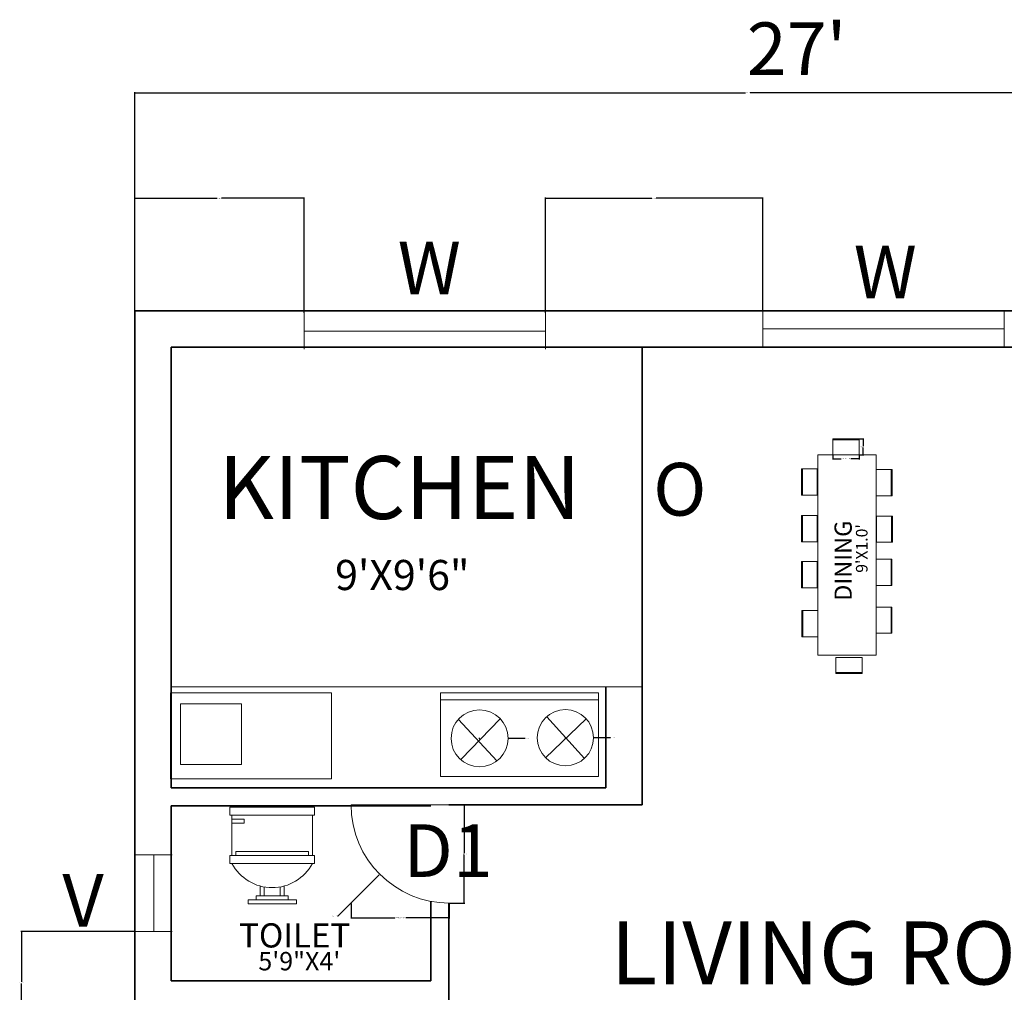
# Model space of a CAD drawing. Units: inches. Extents: x -26 to 788, y -42 to 505.
# Tile 5 of 9: x -26 to 219, y 262 to 504. Entities that reach past the tile are written whole.
import ezdxf

# ---------------------------------------------------------------- set-up
doc = ezdxf.new("R2010")
doc.units = ezdxf.units.IN
doc.header["$MEASUREMENT"] = 0
for name, color, linetype, lineweight in [('A-ANNO-DIMS', 2, 'Continuous', 18), ('A-ANNO-IDEN', 3, 'Continuous', 18), ('A-AREA-IDEN', 7, 'Continuous', 18), ('A-DOOR', 3, 'Continuous', 18), ('A-EQPM', 8, 'Continuous', 18), ('A-FLOR-FIXT', 9, 'Continuous', 18), ('A-FURN', 8, 'Continuous', 18), ('A-GLAZ', 4, 'Continuous', 18), ('A-WALL', 7, 'Continuous', 35)]:
    doc.layers.add(name, color=color, linetype=linetype, lineweight=lineweight)
doc.styles.get("Standard").update_dxf_attribs({"font": 'arial.ttf'})
doc.dimstyles.get("Standard").update_dxf_attribs({"dimtxt": 0.18, "dimasz": 0.18, "dimexe": 0.18, "dimexo": 0.0625, "dimgap": 0.09, "dimtad": 0, "dimtih": 1, "dimtoh": 1, "dimdec": 4, "dimzin": 0, "dimdsep": 46, "dimtxsty": 'Standard', "dimcen": 0.09, "dimadec": 0, "dimazin": 0, "dimtfac": 1, "dimtdec": 4, "dimtofl": 0, "dimtmove": 0, "dimatfit": 3, "dimfxl": 1, "dimtolj": 1, "dimtzin": 0, "dimarcsym": 0})

# ---------------------------------------------------------------- blocks, each defined once
blk = doc.blocks.new('*U2')
for p, q in [((-10, 22), (-10, 12)), ((-10, 21), (-7, 21)), ((-7, 20), (-10, 20)), ((-7, 21), (-7, 20)), ((10, 12), (10, 22)), ((9, 13), (-9, 13)), ((-9, 13), (-9, 12)), ((9, 12), (9, 13)), ((10.5, 12), (-10.5, 12)), ((-10.5, 10), (-10.5, 12)), ((10.5, 10), (-10.5, 10)), ((10.5, 12), (10.5, 10)), ((-3, 4.4065), (-3, 2)), ((-2, 2), (-2, 4.1658)), ((2, 4.1658), (2, 2)), ((3, 2), (3, 4.4065)), ((4, 2), (-4, 2)), ((-4, 2), (-4, 1)), ((4, 1), (4, 2))]:
    blk.add_line(p, q)
for points in [[(10.5, 22), (10.5, 24), (-10.5, 24), (-10.5, 22)], [(6, 0), (6, 1), (-6, 1), (-6, 0)]]:
    blk.add_lwpolyline(points, close=True)
blk.add_arc((0, 15.3333), 11.3333, 208.0725, 331.9275)
blk = doc.blocks.new('*D7')
at = {"layer": 'A-ANNO-DIMS', "color": 0, "lineweight": -2, "transparency": 16777216}
for p, q in [((2.95, 431.18), (2.95, 485.53)), ((3.13, 485.35), (154.6, 485.35)), ((307.27, 485.35), (155.81, 485.35)), ((307.45, 431.18), (307.45, 485.53))]:
    blk.add_line(p, q, dxfattribs=at)
at = {"layer": 'A-ANNO-DIMS', "color": 0, "transparency": 16777216}
for points in [[(3.13, 485.38), (3.13, 485.32), (2.95, 485.35)], [(307.27, 485.38), (307.27, 485.32), (307.45, 485.35)]]:
    blk.add_solid(points, dxfattribs=at)
at = {"layer": 'Defpoints', "color": 0, "transparency": 16777216}
for p in [(307.45, 485.35), (2.95, 431.12), (307.45, 431.12)]:
    blk.add_point(p, dxfattribs=at)
at = {"layer": 'A-ANNO-DIMS', "color": 0, "transparency": 16777216, "insert": (155.2, 485.35), "char_height": 0.18, "attachment_point": 5}
blk.add_mtext('\\A1;304.5000', dxfattribs=at)
blk = doc.blocks.new('WIN-SLIDER-60')
for p, q in [((0, 9), (0, 0)), ((60, 9), (60, 0)), ((0, 4.5), (60, 4.5)), ((60, 4.5), (50.65, 4.5))]:
    blk.add_line(p, q)
blk = doc.blocks.new('VENT-BATH')
for p, q in [((9, 19.08), (0, 19.08)), ((4.5, 19.08), (4.5, 0)), ((9, 0), (0, 0))]:
    blk.add_line(p, q)
blk = doc.blocks.new('DOOR-BATH-B')
blk.add_line((24.41, 24.41), (0, 24.41))
blk.add_arc((24.41, 24.41), 24.41, 180, 270)
blk = doc.blocks.new('CHAIR-DINING')
for points in [[(0, 3.72), (6.52, 3.72), (6.52, 3.95), (0, 3.95)], [(0, 0), (6.52, 0), (6.52, 3.72), (0, 3.72)]]:
    blk.add_lwpolyline(points, close=True)
blk = doc.blocks.new('*D25')
at = {"layer": 'A-ANNO-DIMS', "color": 0, "lineweight": -2, "transparency": 16777216}
for p, q in [((176.36, 395.3), (176.36, 394.21)), ((176.54, 394.39), (178.43, 394.39)), ((182.71, 394.39), (180.82, 394.39)), ((182.89, 395.3), (182.89, 394.21))]:
    blk.add_line(p, q, dxfattribs=at)
at = {"layer": 'A-ANNO-DIMS', "color": 0, "transparency": 16777216}
for points in [[(176.54, 394.42), (176.54, 394.36), (176.36, 394.39)], [(182.71, 394.42), (182.71, 394.36), (182.89, 394.39)]]:
    blk.add_solid(points, dxfattribs=at)
at = {"layer": 'Defpoints', "color": 0, "transparency": 16777216}
for p in [(176.36, 395.37), (182.89, 395.37), (182.89, 394.39)]:
    blk.add_point(p, dxfattribs=at)
at = {"layer": 'A-ANNO-DIMS', "color": 0, "transparency": 16777216, "insert": (179.62, 394.39), "char_height": 0.18, "attachment_point": 5}
blk.add_mtext('\\A1;CHAIR 6.5246 TYP.', dxfattribs=at)
blk = doc.blocks.new('*D26')
at = {"layer": 'A-ANNO-DIMS', "color": 0, "lineweight": -2, "transparency": 16777216}
for p, q in [((182.95, 399.32), (184.04, 399.32)), ((183.86, 399.14), (183.86, 397.52)), ((183.86, 395.55), (183.86, 397.16)), ((182.95, 395.37), (184.04, 395.37))]:
    blk.add_line(p, q, dxfattribs=at)
at = {"layer": 'A-ANNO-DIMS', "color": 0, "transparency": 16777216}
for points in [[(183.83, 399.14), (183.89, 399.14), (183.86, 399.32)], [(183.83, 395.55), (183.89, 395.55), (183.86, 395.37)]]:
    blk.add_solid(points, dxfattribs=at)
at = {"layer": 'Defpoints', "color": 0, "transparency": 16777216}
for p in [(182.89, 399.32), (183.86, 399.32), (182.89, 395.37)]:
    blk.add_point(p, dxfattribs=at)
at = {"layer": 'A-ANNO-DIMS', "color": 0, "transparency": 16777216, "insert": (183.86, 397.34), "char_height": 0.18, "attachment_point": 5}
blk.add_mtext('\\A1;3.9484 TYP.', dxfattribs=at)
blk = doc.blocks.new('*D41')
at = {"layer": 'A-ANNO-DIMS', "color": 0, "lineweight": -2, "transparency": 16777216}
for p, q in [((56.64, 283.9), (56.64, 280.13)), ((81.05, 283.9), (81.05, 280.13)), ((56.82, 280.31), (67.48, 280.31)), ((80.87, 280.31), (70.22, 280.31))]:
    blk.add_line(p, q, dxfattribs=at)
at = {"layer": 'A-ANNO-DIMS', "color": 0, "transparency": 16777216}
for points in [[(56.82, 280.34), (56.82, 280.28), (56.64, 280.31)], [(80.87, 280.34), (80.87, 280.28), (81.05, 280.31)]]:
    blk.add_solid(points, dxfattribs=at)
at = {"layer": 'Defpoints', "color": 0, "transparency": 16777216}
for p in [(56.64, 283.97), (81.05, 283.97), (81.05, 280.31)]:
    blk.add_point(p, dxfattribs=at)
at = {"layer": 'A-ANNO-DIMS', "color": 0, "transparency": 16777216, "insert": (68.85, 280.31), "char_height": 0.18, "attachment_point": 5}
blk.add_mtext('\\A1;DOOR B 24.4074 TYP.', dxfattribs=at)
blk = doc.blocks.new('*D42')
at = {"layer": 'A-ANNO-DIMS', "color": 0, "lineweight": -2, "transparency": 16777216}
for p, q in [((81.11, 308.37), (84.89, 308.37)), ((84.71, 308.19), (84.71, 296.35)), ((84.71, 284.15), (84.71, 295.99)), ((81.11, 283.97), (84.89, 283.97))]:
    blk.add_line(p, q, dxfattribs=at)
at = {"layer": 'A-ANNO-DIMS', "color": 0, "transparency": 16777216}
for points in [[(84.68, 308.19), (84.74, 308.19), (84.71, 308.37)], [(84.68, 284.15), (84.74, 284.15), (84.71, 283.97)]]:
    blk.add_solid(points, dxfattribs=at)
at = {"layer": 'Defpoints', "color": 0, "transparency": 16777216}
for p in [(81.05, 308.37), (84.71, 308.37), (81.05, 283.97)]:
    blk.add_point(p, dxfattribs=at)
at = {"layer": 'A-ANNO-DIMS', "color": 0, "transparency": 16777216, "insert": (84.71, 296.17), "char_height": 0.18, "attachment_point": 5}
blk.add_mtext('\\A1;24.4074 TYP.', dxfattribs=at)
blk = doc.blocks.new('*D53')
at = {"layer": 'A-ANNO-DIMS', "color": 0, "lineweight": -2, "transparency": 16777216}
for p, q in [((2.95, 431.18), (2.95, 459.29)), ((3.13, 459.11), (23.42, 459.11)), ((44.78, 459.11), (24.49, 459.11)), ((44.96, 430.69), (44.96, 459.29))]:
    blk.add_line(p, q, dxfattribs=at)
at = {"layer": 'A-ANNO-DIMS', "color": 0, "transparency": 16777216}
for points in [[(3.13, 459.14), (3.13, 459.08), (2.95, 459.11)], [(44.78, 459.14), (44.78, 459.08), (44.96, 459.11)]]:
    blk.add_solid(points, dxfattribs=at)
at = {"layer": 'Defpoints', "color": 0, "transparency": 16777216}
for p in [(44.96, 459.11), (2.95, 431.12), (44.96, 430.63)]:
    blk.add_point(p, dxfattribs=at)
at = {"layer": 'A-ANNO-DIMS', "color": 0, "transparency": 16777216, "insert": (23.96, 459.11), "char_height": 0.18, "attachment_point": 5}
blk.add_mtext('\\A1;42.0039', dxfattribs=at)
blk = doc.blocks.new('*D54')
at = {"layer": 'A-ANNO-DIMS', "color": 0, "lineweight": -2, "transparency": 16777216}
for p, q in [((104.96, 430.69), (104.96, 459.29)), ((105.14, 459.11), (131.4, 459.11)), ((158.74, 459.11), (132.47, 459.11)), ((158.92, 431.23), (158.92, 459.29))]:
    blk.add_line(p, q, dxfattribs=at)
at = {"layer": 'A-ANNO-DIMS', "color": 0, "transparency": 16777216}
for points in [[(105.14, 459.14), (105.14, 459.08), (104.96, 459.11)], [(158.74, 459.14), (158.74, 459.08), (158.92, 459.11)]]:
    blk.add_solid(points, dxfattribs=at)
at = {"layer": 'Defpoints', "color": 0, "transparency": 16777216}
for p in [(158.92, 459.11), (104.96, 430.63), (158.92, 431.16)]:
    blk.add_point(p, dxfattribs=at)
at = {"layer": 'A-ANNO-DIMS', "color": 0, "transparency": 16777216, "insert": (131.94, 459.11), "char_height": 0.18, "attachment_point": 5}
blk.add_mtext('\\A1;53.9573', dxfattribs=at)
blk = doc.blocks.new('*D60')
at = {"layer": 'A-ANNO-DIMS', "color": 0, "lineweight": -2, "transparency": 16777216}
for p, q in [((3.11, 276.89), (-25.4, 276.89)), ((-25.22, 276.71), (-25.22, 264.36)), ((-25.22, 251.64), (-25.22, 263.99)), ((2.66, 251.46), (-25.4, 251.46))]:
    blk.add_line(p, q, dxfattribs=at)
at = {"layer": 'A-ANNO-DIMS', "color": 0, "transparency": 16777216}
for points in [[(-25.25, 276.71), (-25.19, 276.71), (-25.22, 276.89)], [(-25.25, 251.64), (-25.19, 251.64), (-25.22, 251.46)]]:
    blk.add_solid(points, dxfattribs=at)
at = {"layer": 'Defpoints', "color": 0, "transparency": 16777216}
for p in [(-25.22, 276.89), (3.17, 276.89), (2.73, 251.46)]:
    blk.add_point(p, dxfattribs=at)
at = {"layer": 'A-ANNO-DIMS', "color": 0, "transparency": 16777216, "insert": (-25.22, 264.17), "char_height": 0.18, "attachment_point": 5}
blk.add_mtext('\\A1;25.4255', dxfattribs=at)
blk = doc.blocks.new('*D64')
at = {"layer": 'A-ANNO-DIMS', "color": 0, "lineweight": -2, "transparency": 16777216}
for p, q in [((88.48, 324.91), (88.66, 324.91)), ((88.57, 324.82), (88.57, 325)), ((99.89, 324.91), (95.83, 324.91))]:
    blk.add_line(p, q, dxfattribs=at)
at = {"layer": 'A-ANNO-DIMS', "color": 0, "transparency": 16777216}
blk.add_solid([(95.83, 324.94), (95.83, 324.88), (95.65, 324.91)], dxfattribs=at)
at = {"layer": 'Defpoints', "color": 0, "transparency": 16777216}
for p in [(81.49, 324.91), (95.65, 324.91)]:
    blk.add_point(p, dxfattribs=at)
at = {"layer": 'A-ANNO-DIMS', "color": 0, "transparency": 16777216, "insert": (100.53, 324.91), "char_height": 0.18, "attachment_point": 5}
blk.add_mtext('\\A1;∅14.1538', dxfattribs=at)
blk = doc.blocks.new('*D65')
at = {"layer": 'A-ANNO-DIMS', "color": 0, "lineweight": -2, "transparency": 16777216}
for p, q in [((109.79, 325.06), (109.97, 325.06)), ((109.88, 324.97), (109.88, 325.15)), ((121.07, 325.06), (117.05, 325.06))]:
    blk.add_line(p, q, dxfattribs=at)
at = {"layer": 'A-ANNO-DIMS', "color": 0, "transparency": 16777216}
blk.add_solid([(117.05, 325.09), (117.05, 325.03), (116.87, 325.06)], dxfattribs=at)
at = {"layer": 'Defpoints', "color": 0, "transparency": 16777216}
for p in [(102.89, 325.06), (116.87, 325.06)]:
    blk.add_point(p, dxfattribs=at)
at = {"layer": 'A-ANNO-DIMS', "color": 0, "transparency": 16777216, "insert": (121.7, 325.06), "char_height": 0.18, "attachment_point": 5}
blk.add_mtext('\\A1;∅13.9833', dxfattribs=at)
blk = doc.blocks.new('*D67')
at = {"layer": 'A-ANNO-DIMS', "color": 0, "lineweight": -2, "transparency": 16777216}
for p, q in [((80.96, 308.37), (81.14, 308.37)), ((81.05, 308.28), (81.05, 308.46)), ((53.44, 280.76), (63.66, 290.99)), ((53.26, 280.76), (53.44, 280.76))]:
    blk.add_line(p, q, dxfattribs=at)
at = {"layer": 'A-ANNO-DIMS', "color": 0, "transparency": 16777216}
blk.add_solid([(63.64, 291.01), (63.68, 290.97), (63.79, 291.12)], dxfattribs=at)
at = {"layer": 'Defpoints', "color": 0, "transparency": 16777216}
for p in [(81.05, 308.37), (63.79, 291.12)]:
    blk.add_point(p, dxfattribs=at)
at = {"layer": 'A-ANNO-DIMS', "color": 0, "transparency": 16777216, "insert": (52.44, 280.76), "char_height": 0.18, "attachment_point": 5}
blk.add_mtext('\\A1;2X R24.4074', dxfattribs=at)

msp = doc.modelspace()

# ---------------------------------------------------------------- linework, layer by layer
at = {"layer": 'A-EQPM'}
for p, q in [((78.85143, 334.51728), (118.11677, 334.51728)), ((105.2413, 330.24869), (114.5985, 319.87908)), ((83.30298, 329.62023), (92.81745, 319.32917)), ((93.6824, 329.77734), (84.01066, 319.72196)), ((115.07029, 329.77734), (104.92677, 320.03619))]:
    msp.add_line(p, q, dxfattribs=at)
msp.add_lwpolyline([(78.8556, 336.22802), (118.08773, 336.22802), (118.08773, 315.45463), (78.8556, 315.45463)], close=True, dxfattribs=at)
for centre, radius in [((88.57132, 324.90677), 7.07688), ((109.88058, 325.06388), 6.99163)]:
    msp.add_circle(centre, radius, dxfattribs=at)
at = {"layer": 'A-FLOR-FIXT'}
msp.add_line((11.95497, 337.72642), (128.95497, 337.72642), dxfattribs=at)
for points in [[(11.76865, 336.22802), (51.78543, 336.22802), (51.78543, 314.8667), (11.76865, 314.8667)], [(14.31874, 333.48436), (29.42311, 333.48436), (29.42311, 318.39426), (14.31874, 318.39426)]]:
    msp.add_lwpolyline(points, close=True, dxfattribs=at)
at = {"layer": 'A-FURN'}
msp.add_lwpolyline([(172.60237, 395.39346), (187.08011, 395.39346), (187.08011, 345.57278), (172.60237, 345.57278)], close=True, dxfattribs=at)
at = {"layer": 'A-WALL'}
for p, q in [((2.95497, 2.11777), (2.95497, 431.11777)), ((2.95497, 431.11777), (307.45497, 431.11777)), ((11.95497, 312.61777), (11.95497, 422.11777)), ((11.95497, 422.11777), (128.95497, 422.11777)), ((128.95497, 308.37421), (128.95497, 422.11777)), ((128.95497, 422.11777), (235.45497, 422.11777)), ((119.95497, 312.61777), (119.95497, 337.72642)), ((11.95497, 312.61777), (80.95497, 312.61777)), ((80.95497, 312.61777), (119.97034, 312.61777)), ((80.95497, 308.37421), (128.95497, 308.37421)), ((11.95497, 308.11777), (76.45497, 308.11777)), ((11.95497, 264.61777), (11.95497, 308.11777)), ((76.45497, 264.61777), (76.45497, 284.40319)), ((80.95497, 195.61777), (80.95497, 283.96697)), ((11.95497, 264.61777), (76.45497, 264.61777))]:
    msp.add_line(p, q, dxfattribs=at)

# ---------------------------------------------------------------- block references
at = {"layer": 'A-DOOR'}
msp.add_blockref('DOOR-BATH-B', (56.642, 283.967), dxfattribs=at)
at = {"layer": 'A-FLOR-FIXT'}
msp.add_blockref('*U2', (37.05412, 283.81026), dxfattribs=at)
at = {"layer": 'A-FURN'}
msp.add_blockref('CHAIR-DINING', (176.361, 395.367), dxfattribs=at)
for p, rotation in [((172.4693, 385.36498), 90.0000000000003), ((187.08486, 391.70892), 270.0000000000007), ((172.4693, 373.77305), 90.00000000000067), ((187.19863, 380.15671), 270), ((187.05713, 369.41298), 270.0000000000007), ((172.4693, 362.32249), 90.00000000000067), ((187.05713, 357.53832), 270.0000000000007), ((172.6108, 350.1651), 90.00000000000095), ((183.5858, 344.99557), 180)]:
    msp.add_blockref('CHAIR-DINING', p, dxfattribs=dict(at, rotation=rotation))
at = {"layer": 'A-GLAZ'}
for name, p in [('WIN-SLIDER-60', (44.95844, 421.63218)), ('WIN-SLIDER-60', (158.9157, 422.16419)), ('VENT-BATH', (3.17247, 276.88611))]:
    msp.add_blockref(name, p, dxfattribs=at)

# ---------------------------------------------------------------- texts
at = {"layer": 'A-ANNO-DIMS'}
msp.add_text("27'", height=13.093175, dxfattribs=at).set_placement((154.94713, 489.7308))
at = {"layer": 'A-ANNO-IDEN'}
for s, height, p in [('W', 13.09317, (68.24105, 435.21429)), ('W', 13.09317, (181.51044, 434.27907)), ('O', 13.09317, (131.68912, 380.25852)), ('D1', 13.093175, (69.64848, 290.46019)), ('V', 13.09317, (-15.07276, 278.0963))]:
    msp.add_text(s, height=height, dxfattribs=at).set_placement(p)
at = {"layer": 'A-AREA-IDEN'}
for s, height, p in [('KITCHEN', 15.645019, (23.69366, 379.42261)), ('9\'X9\'6"', 7.483862, (52.69068, 361.75679)), ('TOILET', 6.011917, (28.84451, 272.93248)), ('LIVING ROOM', 15.6450193, (121.09986, 263.74771)), ('5\'9"X4\'', 4.56659, (33.60912, 267.24823))]:
    msp.add_text(s, height=height, dxfattribs=at).set_placement(p)
for s, height, p in [('DINING', 4.282665, (181.02004, 359.08002)), ("9'X1.0'", 2.879999, (184.95026, 366.05532))]:
    msp.add_text(s, height=height, rotation=90, dxfattribs=at).set_placement(p)

# ---------------------------------------------------------------- dimensions: what is measured, and where the dimension line sits
at = {"layer": 'A-ANNO-DIMS'}
for base, p1, p2, override, picture, middle in [((307.45497, 485.35153), (2.95497, 431.11777), (307.45497, 431.11777), {"dimclrd": 0, "dimclre": 0, "dimclrt": 0}, '*D7', (155.20497, 485.35153)), ((44.95884, 459.11412), (2.95497, 431.11777), (44.95884, 430.6321), {"dimdec": 4, "dimlfac": 1, "dimrnd": 0, "dimzin": 0, "dimdsep": 46, "dimlunit": 2}, '*D53', (23.9569, 459.11412)), ((158.9161, 459.11412), (104.95884, 430.6321), (158.9161, 431.16412), {"dimdec": 4, "dimlfac": 1, "dimrnd": 0, "dimzin": 0, "dimdsep": 46, "dimlunit": 2}, '*D54', (131.93747, 459.11412))]:
    dim = msp.add_linear_dim(base=base, p1=p1, p2=p2, dimstyle='Standard', override=override, dxfattribs=at)
    dim.commit()
    dim.dimension.update_dxf_attribs({"geometry": picture, "text_midpoint": middle})
for base, p1, p2, picture, middle in [((183.86448, 399.31546), (182.88579, 395.36705), (182.88579, 399.31546), '*D26', (183.86448, 397.34125)), ((84.71095, 308.37421), (81.04983, 283.96678), (81.04983, 308.37421), '*D42', (84.71095, 296.1705))]:
    dim = msp.add_linear_dim(base=base, p1=p1, p2=p2, angle=90, text='<> TYP.', dimstyle='Standard', override={"dimdec": 4, "dimlfac": 1, "dimrnd": 0, "dimzin": 0, "dimdsep": 46, "dimlunit": 2}, dxfattribs=at)
    dim.commit()
    dim.dimension.update_dxf_attribs({"geometry": picture, "text_midpoint": middle})
for base, p1, p2, text, picture, middle in [((182.885794, 394.388362), (176.361238, 395.367046), (182.885794, 395.367046), 'CHAIR <> TYP.', '*D25', (179.623516, 394.388362)), ((81.04983, 280.30567), (56.64241, 283.96678), (81.04983, 283.96678), 'DOOR B <> TYP.', '*D41', (68.84612, 280.30567))]:
    dim = msp.add_linear_dim(base=base, p1=p1, p2=p2, text=text, dimstyle='Standard', override={"dimdec": 4, "dimlfac": 1, "dimrnd": 0, "dimzin": 0, "dimdsep": 46, "dimlunit": 2}, dxfattribs=at)
    dim.commit()
    dim.dimension.update_dxf_attribs({"geometry": picture, "text_midpoint": middle})
for p1, p2, picture, middle in [((81.49444, 324.90653), (95.6482, 324.907), '*D64', (99.89432, 324.90714)), ((102.88895, 325.06377), (116.87221, 325.064), '*D65', (121.06719, 325.06407))]:
    dim = msp.add_diameter_dim_2p(p1=p1, p2=p2, dimstyle='Standard', override={"dimdec": 4, "dimlfac": 1, "dimrnd": 0, "dimzin": 0, "dimdsep": 46, "dimlunit": 2}, dxfattribs=at)
    dim.commit()
    dim.dimension.update_dxf_attribs({"geometry": picture, "text_midpoint": middle, "dimtype": 163})
dim = msp.add_radius_dim(center=(81.04983, 308.37421), mpoint=(63.79086, 291.11586), text='2X <>', dimstyle='Standard', override={"dimdec": 4, "dimlfac": 1, "dimrnd": 0, "dimzin": 0, "dimdsep": 46, "dimlunit": 2}, dxfattribs=at)
dim.commit()
dim.dimension.update_dxf_attribs({"geometry": '*D67', "text_midpoint": (52.44125, 280.76086), "dimtype": 164})
dim = msp.add_linear_dim(base=(-25.22286, 276.88608), p1=(2.72715, 251.46056), p2=(3.17262, 276.88608), angle=90, dimstyle='Standard', override={"dimdec": 4, "dimlfac": 1, "dimrnd": 0, "dimzin": 0, "dimdsep": 46, "dimlunit": 2}, dxfattribs=at)
dim.commit()
dim.dimension.update_dxf_attribs({"geometry": '*D60', "text_midpoint": (-25.22285, 264.17332)})

doc.saveas('drawing.dxf')
